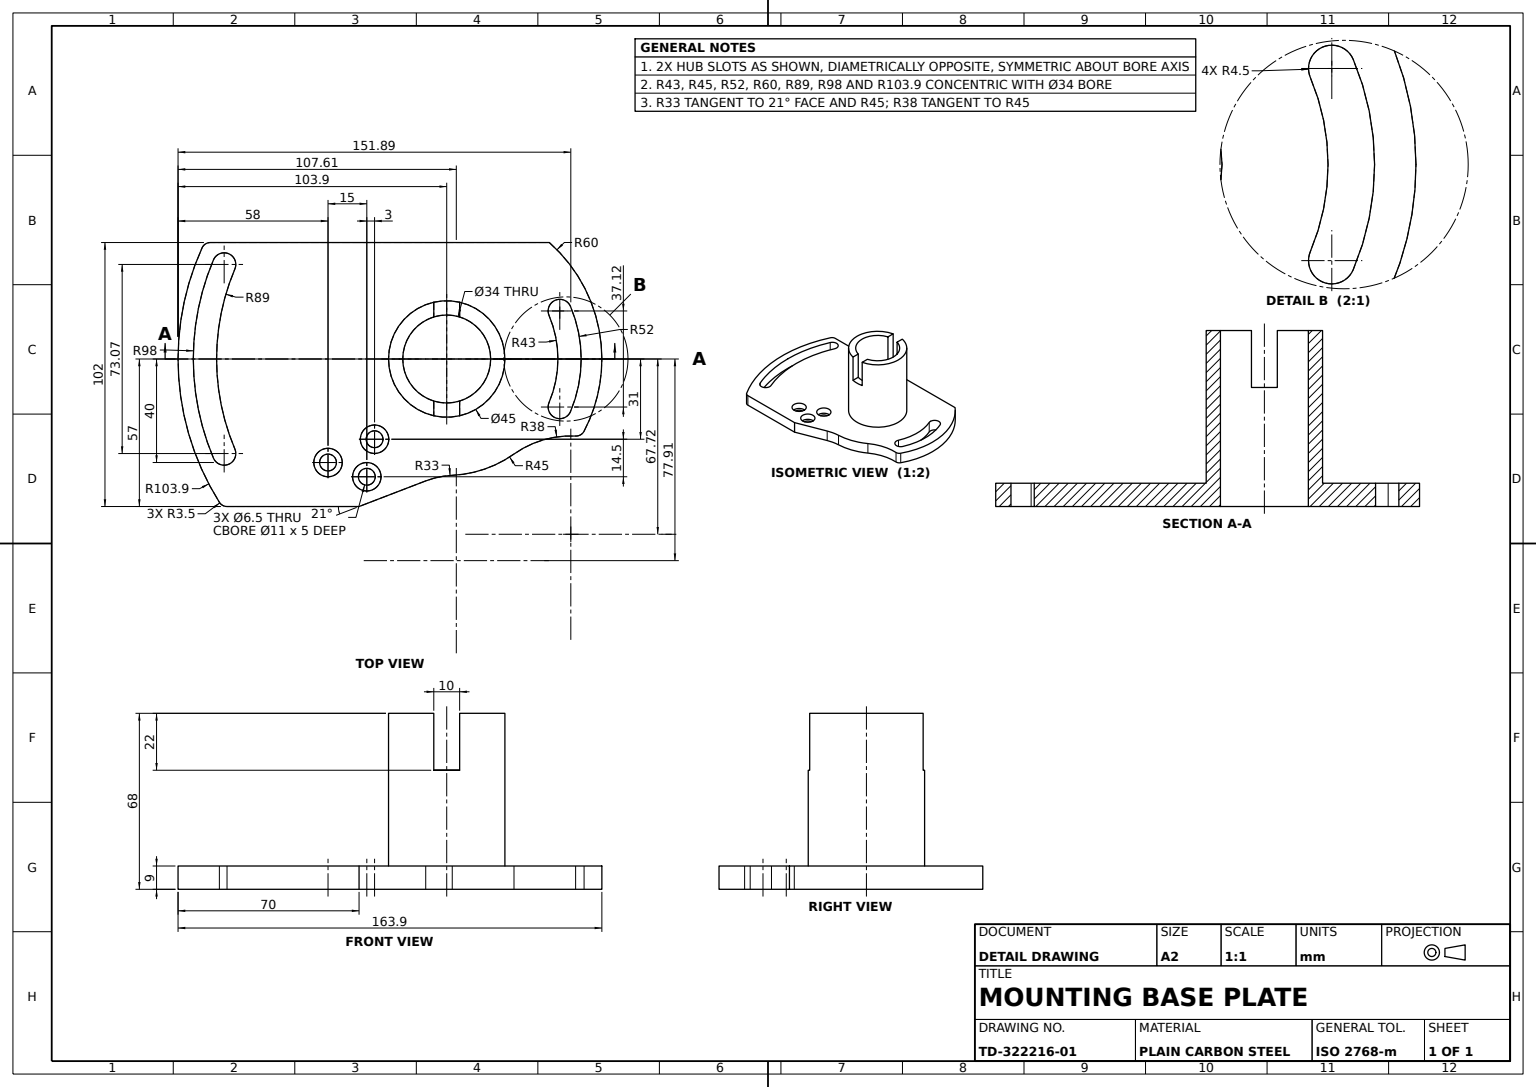
from build123d import *

# Parameters (mm, degrees)
CAM_PLATE_9MM_DEPTH                = 9
ARC_SLOTS_REACH                    = 120.85
COUNTERBORED_HOLES_6_5_D           = 6.5
COUNTERBORED_HOLES_6_5_CBORE_D     = 11
COUNTERBORED_HOLES_6_5_CBORE_DEPTH = 5
HUB_PROFILE_45_R                   = 22.5
HUB_45_DEPTH                       = 59
HUB_BORE_PROFILE_34_R              = 17
HUB_BORE_34_DEPTH                  = 137.631658118
HUB_SLOTS_PROFILE_W                = 45
HUB_SLOTS_PROFILE_H                = 10
HUB_SLOTS_10MM_DEPTH               = 22


with BuildPart() as part:
    # Cam Plate Profile → Cam Plate 9mm (new body)
    with BuildSketch(Plane(origin=(0, 0, 0), x_dir=(1, 0, 0), z_dir=(0, 1, 0))):
        with BuildLine():
            Line((-45, 39.685663216), (-45, -91.421605761))
            ThreePointArc((-45, -91.421605761), (-44.442235206, -93.317193267), (-42.946713147, -94.60861393))
            ThreePointArc((-42.946713147, -94.60861393), (7.05252971, -103.660367666), (55.365039841, -87.919977044))
            ThreePointArc((55.365039841, -87.919977044), (56.564118098, -86.649786254), (57, -84.958283881))
            Line((57, -84.958283881), (57, -33.9))
            Line((57, -33.9), (47.103714625, -8.119295188))
            ThreePointArc((47.103714625, -8.119295188), (45.616562216, -3.076454346), (44.949155019, 2.138565661))
            ThreePointArc((44.949155019, 2.138565661), (42.542307371, 14.668063387), (36.715662651, 26.01845722))
            ThreePointArc((36.715662651, 26.01845722), (31.239721897, 37.350552414), (29.765554185, 49.849717914))
            ThreePointArc((29.765554185, 49.849717914), (29.308643796, 51.757455991), (27.897091162, 53.119715451))
            ThreePointArc((27.897091162, 53.119715451), (-10.874089044, 59.005983191), (-45, 39.685663216))
        make_face()
    extrude(amount=CAM_PLATE_9MM_DEPTH)

    # Arc Slots Profile → Arc Slots (cut, up to next)
    with BuildSketch(Plane(origin=(0, 9, 0), x_dir=(1, 0, 0), z_dir=(0, 1, 0)), mode=Mode.PRIVATE) as arc_slots_sk1:
        with BuildLine():
            ThreePointArc((20.318018681, 47.86625238), (0, 52), (-20.318018681, 47.86625238))
            ThreePointArc((-20.318018681, 47.86625238), (-22.702000444, 41.965690461), (-16.801438525, 39.581708698))
            ThreePointArc((-16.801438525, 39.581708698), (0, 43), (16.801438525, 39.581708698))
            ThreePointArc((16.801438525, 39.581708698), (22.702000444, 41.965690461), (20.318018681, 47.86625238))
        make_face()
    arc_slots_tool1 = extrude(arc_slots_sk1.sketch, amount=-ARC_SLOTS_REACH, mode=Mode.PRIVATE) & part.part
    # Arc Slots Profile → Arc Slots (cut, up to next)
    with BuildSketch(Plane(origin=(0, 9, 0), x_dir=(1, 0, 0), z_dir=(0, 1, 0)), mode=Mode.PRIVATE) as arc_slots_sk2:
        with BuildLine():
            ThreePointArc((-38.291650592, -90.209475638), (0, -98), (38.291650592, -90.209475638))
            ThreePointArc((38.291650592, -90.209475638), (40.675632354, -84.30891372), (34.775070436, -81.924931957))
            ThreePointArc((34.775070436, -81.924931957), (0, -89), (-34.775070436, -81.924931957))
            ThreePointArc((-34.775070436, -81.924931957), (-40.675632354, -84.30891372), (-38.291650592, -90.209475638))
        make_face()
    arc_slots_tool2 = extrude(arc_slots_sk2.sketch, amount=-ARC_SLOTS_REACH, mode=Mode.PRIVATE) & part.part
    add(arc_slots_tool1.solids().sort_by_distance((0, 9, -45.841951))[0], mode=Mode.SUBTRACT)
    add(arc_slots_tool2.solids().sort_by_distance((0, 9, 90.583722))[0], mode=Mode.SUBTRACT)

    # Counterbored Holes Ø6.5 (through all)
    with Locations(Plane(origin=(31, 9, 27.9), x_dir=(0, 0, 1), z_dir=(0, 1, 0))):
        with Locations((0, 0), (3, 14.5), (18, 9)):
            CounterBoreHole(COUNTERBORED_HOLES_6_5_D / 2, COUNTERBORED_HOLES_6_5_CBORE_D / 2, COUNTERBORED_HOLES_6_5_CBORE_DEPTH)

    # Hub Profile Ø45 → Hub Ø45 (add)
    with BuildSketch(Plane(origin=(0, 9, 0), x_dir=(1, 0, 0), z_dir=(0, 1, 0))):
        with Locations(Location((0, 0, 0), (0, 0, 90))):
            Circle(HUB_PROFILE_45_R)
    extrude(amount=HUB_45_DEPTH)

    # Hub Bore Profile Ø34 → Hub Bore Ø34 (cut, through all)
    with BuildSketch(Plane(origin=(0, 68, 0), x_dir=(1, 0, 0), z_dir=(0, 1, 0))):
        with Locations(Location((0, 0, 0), (0, 0, 270))):
            Circle(HUB_BORE_PROFILE_34_R)
    extrude(amount=-HUB_BORE_34_DEPTH, mode=Mode.SUBTRACT)

    # Hub Slots Profile → Hub Slots 10mm (cut)
    with BuildSketch(Plane(origin=(0, 68, 0), x_dir=(1, 0, 0), z_dir=(0, 1, 0))):
        Rectangle(HUB_SLOTS_PROFILE_W, HUB_SLOTS_PROFILE_H)
    extrude(amount=-HUB_SLOTS_10MM_DEPTH, mode=Mode.SUBTRACT)


solid = part.part
